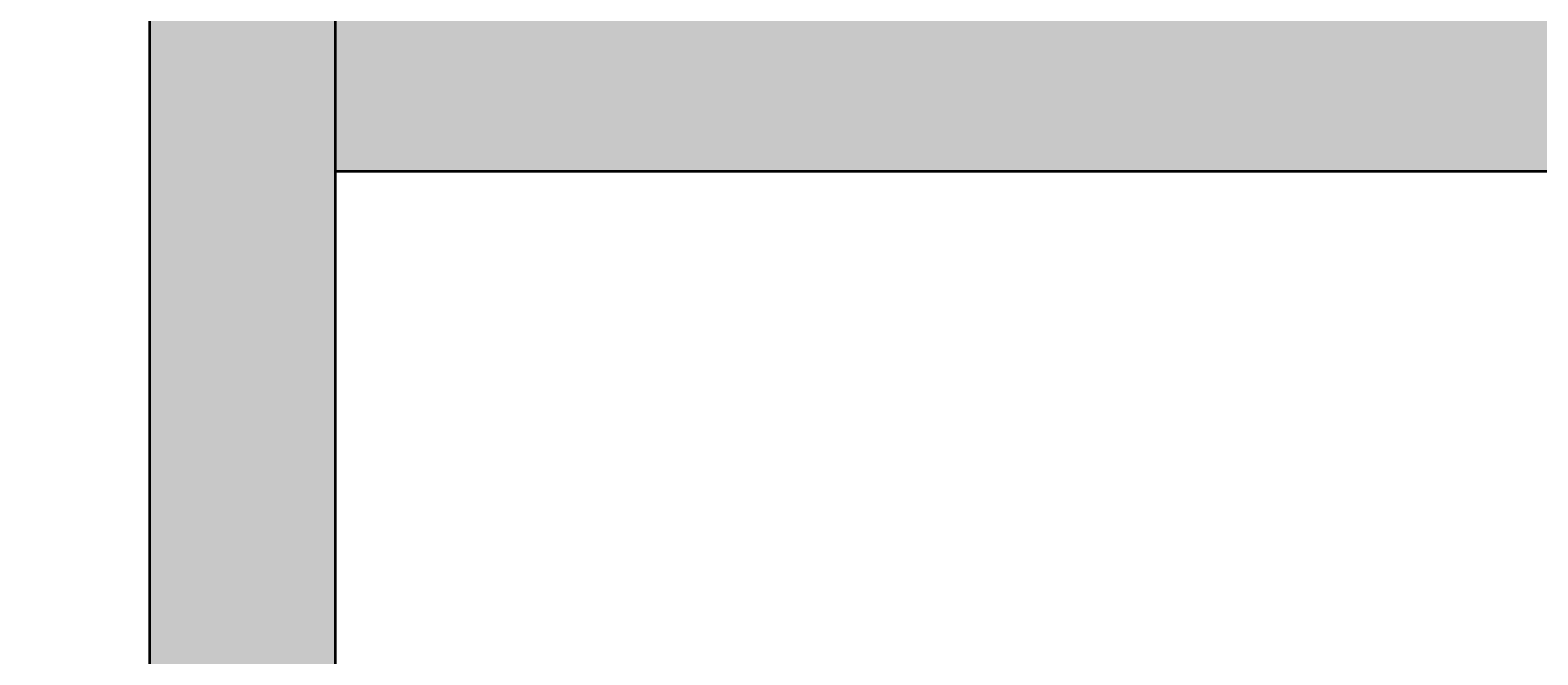
# Model space of a CAD drawing. Units: inches. Extents: x 1998 to 2588, y 1139 to 1977.
# Tile 30 of 134: x 2220 to 2257, y 1506 to 1522. Entities that reach past the tile are written whole.
import ezdxf

# ---------------------------------------------------------------- set-up
doc = ezdxf.new("R2010")
doc.units = ezdxf.units.IN
for name, color, linetype, lineweight in [('A-ANNO-DIMS', 2, 'Continuous', 18), ('A-WALL-PATT', 252, 'Continuous', 13), ('WALL', 200, 'Continuous', 35)]:
    doc.layers.add(name, color=color, linetype=linetype, lineweight=lineweight)
doc.styles.get("Standard").update_dxf_attribs({"font": 'arial.ttf'})
doc.dimstyles.get("Standard").update_dxf_attribs({"dimtxt": 0.18, "dimasz": 0.18, "dimexe": 0.18, "dimexo": 0.0625, "dimgap": 0.09, "dimtad": 0, "dimtih": 1, "dimtoh": 1, "dimdec": 4, "dimzin": 0, "dimdsep": 46, "dimtxsty": 'Standard', "dimcen": 0.09, "dimadec": 0, "dimazin": 0, "dimtfac": 1, "dimtdec": 4, "dimtofl": 0, "dimtmove": 0, "dimatfit": 3, "dimfxl": 1, "dimtolj": 1, "dimtzin": 0, "dimarcsym": 0})

# ---------------------------------------------------------------- blocks, each defined once
blk = doc.blocks.new('*D41')
at = {"layer": 'A-ANNO-DIMS', "color": 0, "lineweight": -2, "transparency": 16777216}
for p, q in [((2227.473, 1588.67), (2227.473, 1138.602)), ((2287.473, 1588.67), (2287.473, 1138.602)), ((2227.653, 1138.782), (2257.254, 1138.782)), ((2287.293, 1138.782), (2257.692, 1138.782))]:
    blk.add_line(p, q, dxfattribs=at)
at = {"layer": 'A-ANNO-DIMS', "color": 0, "transparency": 16777216}
for points in [[(2227.653, 1138.812), (2227.653, 1138.752), (2227.473, 1138.782)], [(2287.293, 1138.812), (2287.293, 1138.752), (2287.473, 1138.782)]]:
    blk.add_solid(points, dxfattribs=at)
at = {"layer": 'Defpoints', "color": 0, "transparency": 16777216}
for p in [(2227.473, 1588.732), (2287.473, 1588.732), (2287.473, 1138.782)]:
    blk.add_point(p, dxfattribs=at)
at = {"layer": 'A-ANNO-DIMS', "color": 0, "transparency": 16777216, "insert": (2257.473, 1138.782), "char_height": 0.18, "attachment_point": 5}
blk.add_mtext('\\A1;60', dxfattribs=at)

msp = doc.modelspace()

# ---------------------------------------------------------------- hatches: boundary and pattern name
at = {"layer": 'A-WALL-PATT'}
h = msp.add_hatch(color=256, dxfattribs=at)
h.dxf.hatch_style = 1
h.paths.add_polyline_path([(2222.9729, 1888.7324), (2099.4125, 1888.7324), (2099.4125, 1879.7324), (2222.9729, 1879.7324)])
h.paths.add_polyline_path([(2096.9729, 1868.3278), (2087.9729, 1868.3278), (2087.9729, 1775.637), (2096.9729, 1775.637)])
h.paths.add_polyline_path([(2227.4729, 1868.3278), (2222.9729, 1868.3278), (2222.9729, 1774.3318), (2227.4729, 1774.3318)])
h.paths.add_polyline_path([(2188.3019, 1759.7324), (2138.6074, 1759.7324), (2099.4125, 1759.7324), (2099.4125, 1755.2324), (2176.9729, 1755.2324), (2188.3019, 1755.2324)])
h.paths.add_polyline_path([(2087.9729, 1759.7324), (2059.4729, 1759.7324), (2059.4729, 1702.7324), (2087.9729, 1702.7324), (2087.9729, 1707.2324), (2063.9729, 1707.2324), (2063.9729, 1755.2324), (2087.9729, 1755.2324)])
h.paths.add_polyline_path([(2096.9729, 1755.2324), (2087.9729, 1755.2324), (2087.9729, 1707.2324), (2096.9729, 1707.2324)])
h.paths.add_polyline_path([(2187.0461, 1707.2324), (2105.9729, 1707.2324), (2096.9729, 1707.2324), (2087.9729, 1707.2324), (2087.9729, 1702.7324), (2105.9729, 1702.7324), (2114.9729, 1702.7324), (2187.0461, 1702.7324)])
h.paths.add_polyline_path([(2181.4729, 1719.2028), (2176.9729, 1719.2028), (2176.9729, 1707.2324), (2181.4729, 1707.2324)])
h.paths.add_polyline_path([(2216.0332, 1588.7324), (2114.9729, 1588.7324), (2105.9729, 1588.7324), (2105.9729, 1584.2324), (2216.0332, 1584.2324)])
h.paths.add_polyline_path([(2077.691, 1588.7324), (2061.4729, 1588.7324), (2061.4729, 1584.2324), (2077.691, 1584.2324)])
h.paths.add_polyline_path([(2105.9729, 1588.7324), (2098.0956, 1588.7324), (2098.0956, 1584.2324), (2105.9729, 1584.2324)])
h.paths.add_polyline_path([(2114.9729, 1596.2642), (2110.1012, 1596.2642), (2105.9729, 1596.2642), (2105.9729, 1588.7324), (2114.9729, 1588.7324)])
h.paths.add_polyline_path([(2114.9729, 1584.2324), (2105.9729, 1584.2324), (2105.9729, 1580.249), (2110.1012, 1580.249), (2114.9729, 1580.249)])
h.paths.add_polyline_path([(2114.9729, 1547.7716), (2110.1012, 1547.7716, -0.0318759), (2105.9729, 1548.035), (2105.9729, 1470.2324), (2108.3775, 1470.2324), (2108.3775, 1465.7324), (2186.2943, 1465.7324), (2186.2943, 1470.2324), (2114.9729, 1470.2324)])
h.paths.add_polyline_path([(2227.4729, 1584.2324), (2222.9729, 1584.2324), (2222.9729, 1486.137), (2227.4729, 1486.137)])
h.paths.add_polyline_path([(2295.4138, 1593.2324), (2227.4729, 1593.2324), (2227.4729, 1588.7324), (2295.4138, 1588.7324), (2295.4138, 1591.8729)])
h.paths.add_polyline_path([(2345.9729, 1627.1165), (2341.4729, 1627.1165), (2341.4729, 1593.2324), (2337.2869, 1593.2324), (2337.2869, 1591.8729), (2337.2869, 1588.7324), (2345.9729, 1588.7324)])
h.paths.add_polyline_path([(2291.9729, 1588.7324), (2287.4729, 1588.7324), (2287.4729, 1522.7324), (2291.9729, 1522.7324)])
h.paths.add_polyline_path([(2291.9729, 1522.7324), (2287.4729, 1522.7324), (2227.4729, 1522.7324), (2227.4729, 1518.2324), (2291.9729, 1518.2324)])
h.paths.add_polyline_path([(2295.7347, 1519.5919), (2295.7347, 1522.7324), (2291.9729, 1522.7324), (2291.9729, 1518.2324), (2295.7347, 1518.2324)])
h.paths.add_polyline_path([(2345.9729, 1522.7324), (2337.6078, 1522.7324), (2337.6078, 1519.5919), (2337.6078, 1518.2324), (2341.4729, 1518.2324), (2341.4729, 1488.5616), (2345.9729, 1488.5616)])
h.paths.add_polyline_path([(2345.9729, 1468.1569), (2341.4729, 1468.1569), (2341.4729, 1374.2324), (2227.4729, 1374.2324), (2227.4729, 1369.7324), (2345.9729, 1369.7324)])
h.paths.add_polyline_path([(2345.9729, 1369.7324), (2341.4729, 1369.7324), (2341.4729, 1362.2324), (2345.9729, 1362.2324)])
h.paths.add_polyline_path([(2345.9729, 1317.7324), (2345.9729, 1322.2324), (2341.4729, 1322.2324), (2341.4729, 1285.137), (2345.9729, 1285.137)], flags=17)
h.paths.add_polyline_path([(2356.2096, 1322.2324), (2345.9729, 1322.2324), (2345.9729, 1317.7324), (2356.2096, 1317.7324), (2356.2096, 1319.3088)], flags=17)
h.paths.add_polyline_path([(2393.9729, 1322.2324), (2375.6999, 1322.2324), (2375.6999, 1319.3088, -0.0202458), (2375.636, 1317.7324), (2393.9729, 1317.7324)], flags=17)
h.paths.add_polyline_path([(2398.4729, 1322.2324), (2393.9729, 1322.2324), (2393.9729, 1317.7324), (2393.9729, 1237.7324), (2345.9729, 1237.7324), (2345.9729, 1264.7324), (2341.4729, 1264.7324), (2341.4729, 1228.7324), (2393.9729, 1228.7324), (2482.7412, 1228.7324), (2482.7412, 1237.7324), (2398.4729, 1237.7324), (2398.4729, 1297.1029)])
h.paths.add_polyline_path([(2398.4729, 1362.2324), (2393.9729, 1362.2324), (2393.9729, 1357.7324), (2398.4729, 1357.7324)])
h.paths.add_polyline_path([(2345.9729, 1329.7549), (2341.4729, 1329.7549), (2341.4729, 1322.2324), (2345.9729, 1322.2324)])

# ---------------------------------------------------------------- linework, layer by layer
at = {"layer": 'WALL'}
for p, q in [((2227.4729, 1588.7324), (2227.4729, 1486.137)), ((2222.9729, 1584.2324), (2222.9729, 1486.137)), ((2227.4729, 1518.2324), (2291.9729, 1518.2324)), ((2227.4729, 1518.2324), (2296.6507, 1518.2324))]:
    msp.add_line(p, q, dxfattribs=at)

# ---------------------------------------------------------------- dimensions: what is measured, and where the dimension line sits
at = {"layer": 'A-ANNO-DIMS'}
dim = msp.add_linear_dim(base=(2287.4729, 1138.7824), p1=(2227.4729, 1588.7324), p2=(2287.4729, 1588.7324), dimstyle='Standard', override={"dimdec": 0, "dimlfac": 1, "dimrnd": 0, "dimzin": 0, "dimdsep": 46, "dimlunit": 2}, dxfattribs=at)
dim.commit()
dim.dimension.update_dxf_attribs({"geometry": '*D41', "text_midpoint": (2257.4729, 1138.7824)})

doc.saveas('drawing.dxf')
